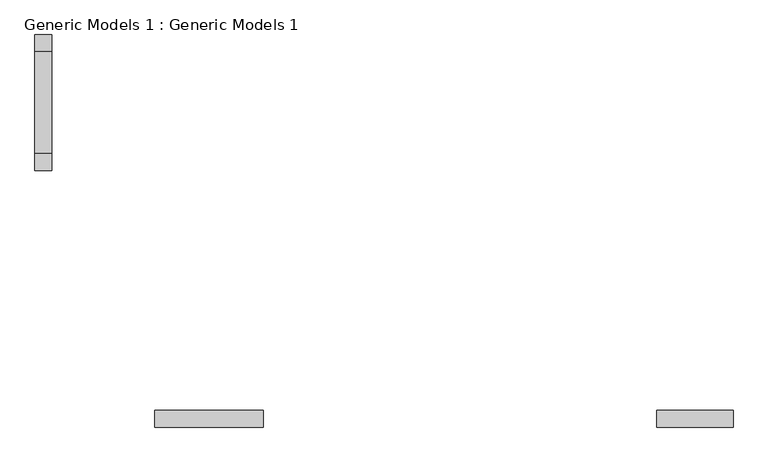
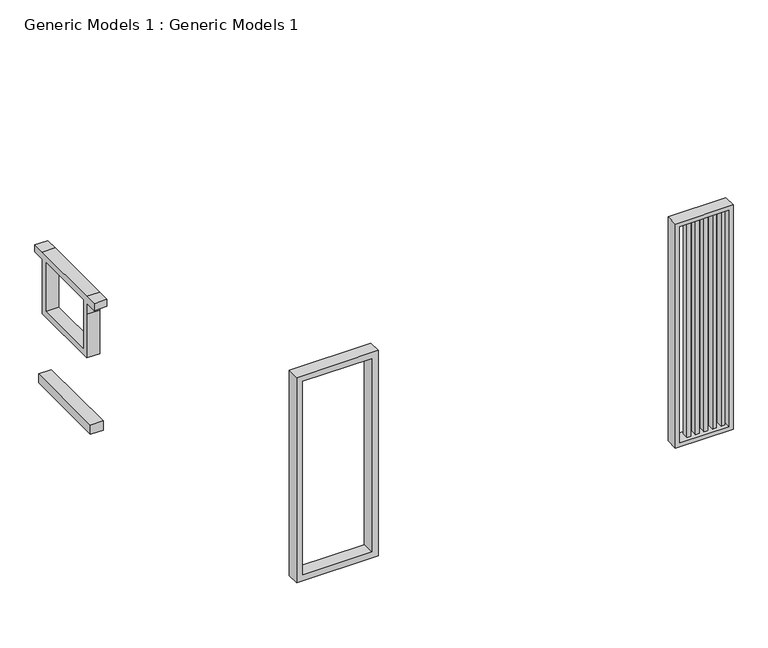
"""IFC4 building model written with IfcOpenShell, lengths in millimetres: proxy geometry, Generic Models 1 : Generic Models 1."""

from ifc_helpers import new_model, si_unit, frame, origin, place, context, project, spatial, polyline, outline, extrude, source, transform, mapped, element, save


def generic_models_1_generic_models_1_10505d45(model_context):
    return source(origin(), model_context, "Body", "SweptSolid", [
        extrude(outline(polyline([(-3104.0178125, 1507.4022755), (-3013.7164923, 1507.4022755), (-3013.7164923, 1352.2634775), (-3104.0178125, 1352.2634775), (-3104.0178125, 1507.4022755)])), frame((0.0, 0.0, 863.6), z_axis=(0.0, 0.0, 1.0), x_axis=(1.0, 0.0, 0.0)), (0.0, 0.0, 1.0), 5435.6),
        extrude(outline(polyline([(-3307.2178125, 1507.4022755), (-3216.9164923, 1507.4022755), (-3216.9164923, 1352.2634775), (-3307.2178125, 1352.2634775), (-3307.2178125, 1507.4022755)])), frame((0.0, 0.0, 863.6), z_axis=(0.0, 0.0, 1.0), x_axis=(1.0, 0.0, 0.0)), (0.0, 0.0, 1.0), 5435.6),
        extrude(outline(polyline([(-3510.4178125, 1507.4022755), (-3420.1164923, 1507.4022755), (-3420.1164923, 1352.2634775), (-3510.4178125, 1352.2634775), (-3510.4178125, 1507.4022755)])), frame((0.0, 0.0, 863.6), z_axis=(0.0, 0.0, 1.0), x_axis=(1.0, 0.0, 0.0)), (0.0, 0.0, 1.0), 5435.6),
        extrude(outline(polyline([(-3713.6178125, 1507.4022755), (-3623.3164923, 1507.4022755), (-3623.3164923, 1352.2634775), (-3713.6178125, 1352.2634775), (-3713.6178125, 1507.4022755)])), frame((0.0, 0.0, 863.6), z_axis=(0.0, 0.0, 1.0), x_axis=(1.0, 0.0, 0.0)), (0.0, 0.0, 1.0), 5435.6),
        extrude(outline(polyline([(-2900.8178125, 1507.4022755), (-2810.5164923, 1507.4022755), (-2810.5164923, 1352.2634775), (-2900.8178125, 1352.2634775), (-2900.8178125, 1507.4022755)])), frame((0.0, 0.0, 863.6), z_axis=(0.0, 0.0, 1.0), x_axis=(1.0, 0.0, 0.0)), (0.0, 0.0, 1.0), 5435.6),
        extrude(outline(polyline([(762.0, -2665.8678125), (6400.8, -2665.8678125), (6400.8, -4037.4678125), (762.0, -4037.4678125), (762.0, -2665.8678125)]), holes=[polyline([(863.6, -3935.8678125), (6299.2, -3935.8678125), (6299.2, -2767.4678125), (863.6, -2767.4678125), (863.6, -3935.8678125)])]), frame((0.0, 1263.416018, 0.0), z_axis=(0.0, 1.0, 0.0), x_axis=(0.0, 0.0, 1.0)), (0.0, 0.0, 1.0), 304.8),
        extrude(outline(polyline([(8007.116018, 3962.4), (6178.316018, 3962.4), (6178.316018, 5054.6), (6178.316018, 5334.0), (5873.516018, 5334.0), (5873.516018, 5511.6269604), (6178.316018, 5511.6269604), (8007.116018, 5511.6269604), (8311.916018, 5511.6269604), (8311.916018, 5334.0), (8007.116018, 5334.0), (8007.116018, 3962.4)]), holes=[polyline([(7854.716018, 4114.8), (7854.716018, 5334.0), (6330.716018, 5334.0), (6330.716018, 4114.8), (7854.716018, 4114.8)])]), frame((-15200.7678125, 0.0, 0.0), z_axis=(1.0, 0.0, 0.0), x_axis=(0.0, 1.0, 0.0)), (0.0, 0.0, 1.0), 304.8),
        extrude(outline(polyline([(-15200.7678125, 6025.916018), (-15200.7678125, 8159.516018), (-14895.9678125, 8159.516018), (-14895.9678125, 6025.916018), (-15200.7678125, 6025.916018)])), frame((0.0, 0.0, 2133.6), z_axis=(0.0, 0.0, 1.0), x_axis=(1.0, 0.0, 0.0)), (0.0, 0.0, 1.0), 228.6),
        extrude(outline(polyline([(530.2676291, -13048.1178125), (530.2676291, -11105.0178125), (5695.95, -11105.0178125), (5695.95, -13048.1178125), (530.2676291, -13048.1178125)]), holes=[polyline([(682.6676291, -12895.7178125), (5543.55, -12895.7178125), (5543.55, -11257.4178125), (682.6676291, -11257.4178125), (682.6676291, -12895.7178125)])]), frame((0.0, 1263.416018, 0.0), z_axis=(0.0, 1.0, 0.0), x_axis=(0.0, 0.0, 1.0)), (0.0, 0.0, 1.0), 304.8),
    ])


if __name__ == "__main__":
    model = new_model("IFC4")
    model_context = context("Model", 3, world=origin())
    ifc_project = project(units=[si_unit("LENGTHUNIT", "METRE", prefix="MILLI")], contexts=[model_context])
    site = spatial("IfcSite", under=ifc_project)
    building = spatial("IfcBuilding", under=site)
    placement = place(None, origin())
    generic_models_1_generic_models_1_shape = generic_models_1_generic_models_1_10505d45(model_context)
    element("IfcBuildingElementProxy", 1, Name="Generic Models 1 : Generic Models 1", ObjectType="Generic Models 1 : Generic Models 1", at=placement, inside=building, context=model_context, shape_type="MappedRepresentation", body=[
        mapped(generic_models_1_generic_models_1_shape, transform((0.0, 0.0, 0.0), x_axis=(1.0, 0.0, 0.0), y_axis=(0.0, 1.0, 0.0), z_axis=(0.0, 0.0, 1.0))),
    ])
    save(model, "model.ifc")

# Revit data of these elements
# Element 1 (IfcBuildingElementProxy, "Generic Models 1 : Generic Models 1")
#   Materials on its faces: "EIFS, Exterior Insulation", "Brick, Common", "Brick, Soldier Course", "Electrical Analytical Loads"
# Materials
#   "EIFS, Exterior Insulation": class "Generic", colour RGB 127 127 127, transparency 0, Description = "EIFS - Exterior Insulation", Cost = 0
#   "Brick, Common": class "Masonry", colour RGB 170 98 104, transparency 0, Description = "Common brick", Cost = 0
#   "Brick, Soldier Course": class "Masonry", colour RGB 170 98 104, transparency 0, Description = "Common brick soldier coursed", Cost = 0
#   "Electrical Analytical Loads": colour RGB 94 94 205, transparency 0.5, Cost = 0
